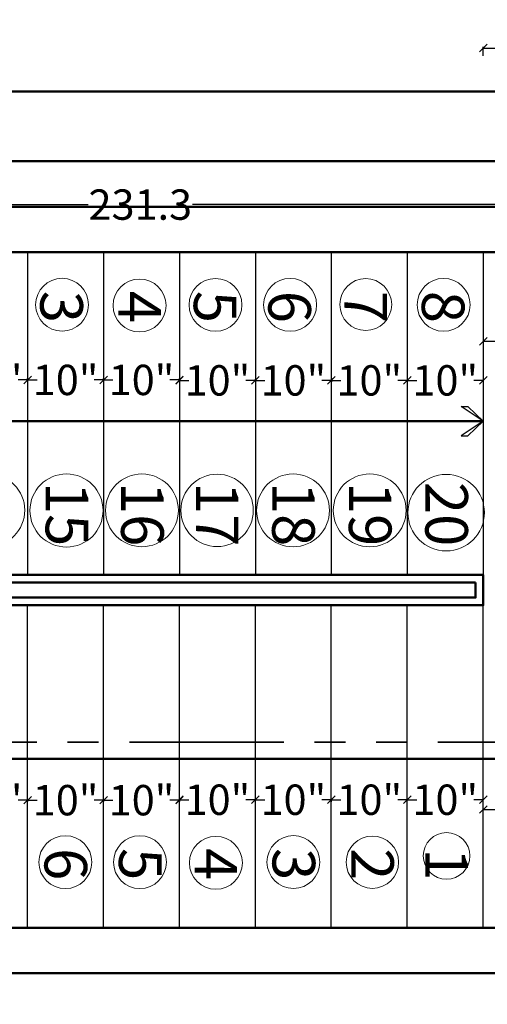
# Model space of a CAD drawing. Units: inches. Extents: x -60 to 284, y -245 to 257.
# Tile 8 of 10: x 99 to 160, y 12 to 141. Entities that reach past the tile are written whole.
import ezdxf

# ---------------------------------------------------------------- set-up
doc = ezdxf.new("R2010")
doc.units = ezdxf.units.IN
doc.header["$LTSCALE"] = 0.8
doc.header["$MEASUREMENT"] = 0
doc.linetypes.add('PHANTOM', pattern=[63.5, 31.75, -6.35, 6.35, -6.35, 6.35, -6.35])
for name, color, linetype, lineweight in [('A-ANNO-DIMS', 2, 'Continuous', 18), ('A-ANNO-SECT', 1, 'PHANTOM', 35), ('A-ANNO-SYMB', 3, 'Continuous', 18), ('A-ANNO-TEXT', 3, 'Continuous', 18), ('A-ANNO-TTLB', 7, 'Continuous', 50), ('A-FLOR-STRS', 4, 'Continuous', 25), ('A-WALL', 7, 'Continuous', 50)]:
    doc.layers.add(name, color=color, linetype=linetype, lineweight=lineweight)
doc.styles.get("Standard").update_dxf_attribs({"font": 'arial.ttf'})
doc.dimstyles.get("Standard").update_dxf_attribs({"dimtxt": 4, "dimasz": 1, "dimexe": 0.18, "dimexo": 0.0625, "dimgap": 0.09, "dimtad": 0, "dimtih": 1, "dimtoh": 1, "dimzin": 0, "dimdsep": 46, "dimlunit": 4, "dimtxsty": 'Standard', "dimblk": 'OBLIQUE', "dimcen": 0.09, "dimadec": 0, "dimazin": 0, "dimtfac": 1, "dimtofl": 0, "dimtmove": 0, "dimatfit": 3, "dimfxl": 1, "dimfxlon": 1, "dimtolj": 1, "dimtzin": 0, "dimarcsym": 0})

# ---------------------------------------------------------------- blocks, each defined once
blk = doc.blocks.new('_Oblique')
at = {"color": 0, "linetype": 'ByBlock', "lineweight": -2}
blk.add_line((-0.5, -0.5), (0.5, 0.5), dxfattribs=at)
blk = doc.blocks.new('*D1')
at = {"layer": 'A-ANNO-DIMS', "color": 0, "lineweight": -2, "ltscale": 0.8, "transparency": 16777216}
for p, q in [((149.94, 37.65), (149.94, 38.72)), ((149.94, 38.54), (151.18, 38.54)), ((159.94, 38.54), (158.69, 38.54)), ((159.94, 37.65), (159.94, 38.72))]:
    blk.add_line(p, q, dxfattribs=at)
at = {"layer": 'Defpoints', "color": 0, "ltscale": 0.8, "transparency": 16777216}
for p in [(149.94, 38.54), (149.94, 37.59), (159.94, 37.59)]:
    blk.add_point(p, dxfattribs=at)
at = {"layer": 'A-ANNO-DIMS', "color": 0, "lineweight": -2, "ltscale": 0.8, "transparency": 16777216, "rotation": 180}
blk.add_blockref('_Oblique', (149.94, 38.54), dxfattribs=at)
at = {"layer": 'A-ANNO-DIMS', "color": 0, "lineweight": -2, "ltscale": 0.8, "transparency": 16777216}
blk.add_blockref('_Oblique', (159.94, 38.54), dxfattribs=at)
at = {"layer": 'A-ANNO-DIMS', "color": 0, "ltscale": 0.8, "transparency": 16777216, "insert": (154.94, 38.54), "char_height": 4, "attachment_point": 5}
blk.add_mtext('\\A1;10"', dxfattribs=at)
blk = doc.blocks.new('*D3')
at = {"layer": 'A-ANNO-DIMS', "color": 0, "lineweight": -2, "ltscale": 0.8, "transparency": 16777216}
for p, q in [((139.94, 38.25), (139.94, 38.72)), ((139.94, 38.54), (141.18, 38.54)), ((149.94, 38.54), (148.69, 38.54)), ((149.94, 38.25), (149.94, 38.72))]:
    blk.add_line(p, q, dxfattribs=at)
at = {"layer": 'Defpoints', "color": 0, "ltscale": 0.8, "transparency": 16777216}
for p in [(139.94, 38.54), (139.94, 38.18), (149.94, 38.18)]:
    blk.add_point(p, dxfattribs=at)
at = {"layer": 'A-ANNO-DIMS', "color": 0, "lineweight": -2, "ltscale": 0.8, "transparency": 16777216, "rotation": 180}
blk.add_blockref('_Oblique', (139.94, 38.54), dxfattribs=at)
at = {"layer": 'A-ANNO-DIMS', "color": 0, "lineweight": -2, "ltscale": 0.8, "transparency": 16777216}
blk.add_blockref('_Oblique', (149.94, 38.54), dxfattribs=at)
at = {"layer": 'A-ANNO-DIMS', "color": 0, "ltscale": 0.8, "transparency": 16777216, "insert": (144.94, 38.54), "char_height": 4, "attachment_point": 5}
blk.add_mtext('\\A1;10"', dxfattribs=at)
blk = doc.blocks.new('*D4')
at = {"layer": 'A-ANNO-DIMS', "color": 0, "lineweight": -2, "ltscale": 0.8, "transparency": 16777216}
for p, q in [((129.94, 38.54), (129.94, 38.72)), ((129.94, 38.54), (131.18, 38.54)), ((139.94, 38.54), (138.69, 38.54)), ((139.94, 38.54), (139.94, 38.72))]:
    blk.add_line(p, q, dxfattribs=at)
at = {"layer": 'Defpoints', "color": 0, "ltscale": 0.8, "transparency": 16777216}
for p in [(129.94, 38.54), (139.94, 38.54), (139.94, 38.48)]:
    blk.add_point(p, dxfattribs=at)
at = {"layer": 'A-ANNO-DIMS', "color": 0, "lineweight": -2, "ltscale": 0.8, "transparency": 16777216, "rotation": 180}
blk.add_blockref('_Oblique', (129.94, 38.54), dxfattribs=at)
at = {"layer": 'A-ANNO-DIMS', "color": 0, "lineweight": -2, "ltscale": 0.8, "transparency": 16777216}
blk.add_blockref('_Oblique', (139.94, 38.54), dxfattribs=at)
at = {"layer": 'A-ANNO-DIMS', "color": 0, "ltscale": 0.8, "transparency": 16777216, "insert": (134.94, 38.54), "char_height": 4, "attachment_point": 5}
blk.add_mtext('\\A1;10"', dxfattribs=at)
blk = doc.blocks.new('*D5')
at = {"layer": 'A-ANNO-DIMS', "color": 0, "lineweight": -2, "ltscale": 0.8, "transparency": 16777216}
for p, q in [((119.94, 38.24), (119.94, 38.72)), ((119.94, 38.54), (121.18, 38.54)), ((129.94, 38.54), (128.69, 38.54)), ((129.94, 38.24), (129.94, 38.72))]:
    blk.add_line(p, q, dxfattribs=at)
at = {"layer": 'Defpoints', "color": 0, "ltscale": 0.8, "transparency": 16777216}
for p in [(119.94, 38.18), (129.94, 38.54), (129.94, 38.18)]:
    blk.add_point(p, dxfattribs=at)
at = {"layer": 'A-ANNO-DIMS', "color": 0, "lineweight": -2, "ltscale": 0.8, "transparency": 16777216, "rotation": 180}
blk.add_blockref('_Oblique', (119.94, 38.54), dxfattribs=at)
at = {"layer": 'A-ANNO-DIMS', "color": 0, "lineweight": -2, "ltscale": 0.8, "transparency": 16777216}
blk.add_blockref('_Oblique', (129.94, 38.54), dxfattribs=at)
at = {"layer": 'A-ANNO-DIMS', "color": 0, "ltscale": 0.8, "transparency": 16777216, "insert": (124.94, 38.54), "char_height": 4, "attachment_point": 5}
blk.add_mtext('\\A1;10"', dxfattribs=at)
blk = doc.blocks.new('*D6')
at = {"layer": 'A-ANNO-DIMS', "color": 0, "lineweight": -2, "ltscale": 0.8, "transparency": 16777216}
for p, q in [((109.94, 38.48), (109.94, 38.3)), ((109.94, 38.48), (111.18, 38.48)), ((119.94, 38.48), (118.69, 38.48)), ((119.94, 38.48), (119.94, 38.3))]:
    blk.add_line(p, q, dxfattribs=at)
at = {"layer": 'Defpoints', "color": 0, "ltscale": 0.8, "transparency": 16777216}
for p in [(109.94, 38.54), (119.94, 38.54), (119.94, 38.48)]:
    blk.add_point(p, dxfattribs=at)
at = {"layer": 'A-ANNO-DIMS', "color": 0, "lineweight": -2, "ltscale": 0.8, "transparency": 16777216, "rotation": 180}
blk.add_blockref('_Oblique', (109.94, 38.48), dxfattribs=at)
at = {"layer": 'A-ANNO-DIMS', "color": 0, "lineweight": -2, "ltscale": 0.8, "transparency": 16777216}
blk.add_blockref('_Oblique', (119.94, 38.48), dxfattribs=at)
at = {"layer": 'A-ANNO-DIMS', "color": 0, "ltscale": 0.8, "transparency": 16777216, "insert": (114.94, 38.48), "char_height": 4, "attachment_point": 5}
blk.add_mtext('\\A1;10"', dxfattribs=at)
blk = doc.blocks.new('*D7')
at = {"layer": 'A-ANNO-DIMS', "color": 0, "lineweight": -2, "ltscale": 0.8, "transparency": 16777216}
for p, q in [((99.94, 38.48), (99.94, 38.66)), ((99.94, 38.48), (101.18, 38.48)), ((109.94, 38.48), (108.69, 38.48)), ((109.94, 38.45), (109.94, 38.66))]:
    blk.add_line(p, q, dxfattribs=at)
at = {"layer": 'Defpoints', "color": 0, "ltscale": 0.8, "transparency": 16777216}
for p in [(99.94, 38.48), (109.94, 38.48), (109.94, 38.39)]:
    blk.add_point(p, dxfattribs=at)
at = {"layer": 'A-ANNO-DIMS', "color": 0, "lineweight": -2, "ltscale": 0.8, "transparency": 16777216, "rotation": 180}
blk.add_blockref('_Oblique', (99.94, 38.48), dxfattribs=at)
at = {"layer": 'A-ANNO-DIMS', "color": 0, "lineweight": -2, "ltscale": 0.8, "transparency": 16777216}
blk.add_blockref('_Oblique', (109.94, 38.48), dxfattribs=at)
at = {"layer": 'A-ANNO-DIMS', "color": 0, "ltscale": 0.8, "transparency": 16777216, "insert": (104.94, 38.48), "char_height": 4, "attachment_point": 5}
blk.add_mtext('\\A1;10"', dxfattribs=at)
blk = doc.blocks.new('*D8')
at = {"layer": 'A-ANNO-DIMS', "color": 0, "lineweight": -2, "ltscale": 0.8, "transparency": 16777216}
for p, q in [((89.94, 38.48), (89.94, 38.66)), ((89.94, 38.48), (91.18, 38.48)), ((99.94, 38.48), (98.69, 38.48)), ((99.94, 38.6), (99.94, 38.3))]:
    blk.add_line(p, q, dxfattribs=at)
at = {"layer": 'Defpoints', "color": 0, "ltscale": 0.8, "transparency": 16777216}
for p in [(89.94, 38.48), (99.94, 38.66), (99.94, 38.48)]:
    blk.add_point(p, dxfattribs=at)
at = {"layer": 'A-ANNO-DIMS', "color": 0, "lineweight": -2, "ltscale": 0.8, "transparency": 16777216, "rotation": 180}
blk.add_blockref('_Oblique', (89.94, 38.48), dxfattribs=at)
at = {"layer": 'A-ANNO-DIMS', "color": 0, "lineweight": -2, "ltscale": 0.8, "transparency": 16777216}
blk.add_blockref('_Oblique', (99.94, 38.48), dxfattribs=at)
at = {"layer": 'A-ANNO-DIMS', "color": 0, "ltscale": 0.8, "transparency": 16777216, "insert": (94.94, 38.48), "char_height": 4, "attachment_point": 5}
blk.add_mtext('\\A1;10"', dxfattribs=at)
blk = doc.blocks.new('*D12')
at = {"layer": 'A-ANNO-DIMS', "color": 0, "lineweight": -2, "ltscale": 0.8, "transparency": 16777216}
for p, q in [((149.94, 94.68), (149.94, 93.61)), ((149.94, 93.79), (151.18, 93.79)), ((159.94, 93.79), (158.69, 93.79)), ((159.94, 94.68), (159.94, 93.61))]:
    blk.add_line(p, q, dxfattribs=at)
at = {"layer": 'Defpoints', "color": 0, "ltscale": 0.8, "transparency": 16777216}
for p in [(149.94, 94.74), (159.94, 94.74), (149.94, 93.79)]:
    blk.add_point(p, dxfattribs=at)
at = {"layer": 'A-ANNO-DIMS', "color": 0, "lineweight": -2, "ltscale": 0.8, "transparency": 16777216, "rotation": 180}
blk.add_blockref('_Oblique', (149.94, 93.79), dxfattribs=at)
at = {"layer": 'A-ANNO-DIMS', "color": 0, "lineweight": -2, "ltscale": 0.8, "transparency": 16777216}
blk.add_blockref('_Oblique', (159.94, 93.79), dxfattribs=at)
at = {"layer": 'A-ANNO-DIMS', "color": 0, "ltscale": 0.8, "transparency": 16777216, "insert": (154.94, 93.79), "char_height": 4, "attachment_point": 5}
blk.add_mtext('\\A1;10"', dxfattribs=at)
blk = doc.blocks.new('*D13')
at = {"layer": 'A-ANNO-DIMS', "color": 0, "lineweight": -2, "ltscale": 0.8, "transparency": 16777216}
for p, q in [((139.94, 94.09), (139.94, 93.61)), ((139.94, 93.79), (141.18, 93.79)), ((149.94, 93.79), (148.69, 93.79)), ((149.94, 94.09), (149.94, 93.61))]:
    blk.add_line(p, q, dxfattribs=at)
at = {"layer": 'Defpoints', "color": 0, "ltscale": 0.8, "transparency": 16777216}
for p in [(139.94, 94.15), (139.94, 93.79), (149.94, 94.15)]:
    blk.add_point(p, dxfattribs=at)
at = {"layer": 'A-ANNO-DIMS', "color": 0, "lineweight": -2, "ltscale": 0.8, "transparency": 16777216, "rotation": 180}
blk.add_blockref('_Oblique', (139.94, 93.79), dxfattribs=at)
at = {"layer": 'A-ANNO-DIMS', "color": 0, "lineweight": -2, "ltscale": 0.8, "transparency": 16777216}
blk.add_blockref('_Oblique', (149.94, 93.79), dxfattribs=at)
at = {"layer": 'A-ANNO-DIMS', "color": 0, "ltscale": 0.8, "transparency": 16777216, "insert": (144.94, 93.79), "char_height": 4, "attachment_point": 5}
blk.add_mtext('\\A1;10"', dxfattribs=at)
blk = doc.blocks.new('*D14')
at = {"layer": 'A-ANNO-DIMS', "color": 0, "lineweight": -2, "ltscale": 0.8, "transparency": 16777216}
for p, q in [((129.94, 93.79), (129.94, 93.97)), ((129.94, 93.79), (131.18, 93.79)), ((139.94, 93.79), (138.69, 93.79)), ((139.94, 93.79), (139.94, 93.61))]:
    blk.add_line(p, q, dxfattribs=at)
at = {"layer": 'Defpoints', "color": 0, "ltscale": 0.8, "transparency": 16777216}
for p in [(129.94, 93.79), (139.94, 93.85), (139.94, 93.79)]:
    blk.add_point(p, dxfattribs=at)
at = {"layer": 'A-ANNO-DIMS', "color": 0, "lineweight": -2, "ltscale": 0.8, "transparency": 16777216, "rotation": 180}
blk.add_blockref('_Oblique', (129.94, 93.79), dxfattribs=at)
at = {"layer": 'A-ANNO-DIMS', "color": 0, "lineweight": -2, "ltscale": 0.8, "transparency": 16777216}
blk.add_blockref('_Oblique', (139.94, 93.79), dxfattribs=at)
at = {"layer": 'A-ANNO-DIMS', "color": 0, "ltscale": 0.8, "transparency": 16777216, "insert": (134.94, 93.79), "char_height": 4, "attachment_point": 5}
blk.add_mtext('\\A1;10"', dxfattribs=at)
blk = doc.blocks.new('*D15')
at = {"layer": 'A-ANNO-DIMS', "color": 0, "lineweight": -2, "ltscale": 0.8, "transparency": 16777216}
for p, q in [((119.94, 94.09), (119.94, 93.61)), ((119.94, 93.79), (121.18, 93.79)), ((129.94, 93.79), (128.69, 93.79)), ((129.94, 94.09), (129.94, 93.61))]:
    blk.add_line(p, q, dxfattribs=at)
at = {"layer": 'Defpoints', "color": 0, "ltscale": 0.8, "transparency": 16777216}
for p in [(119.94, 94.15), (129.94, 94.15), (129.94, 93.79)]:
    blk.add_point(p, dxfattribs=at)
at = {"layer": 'A-ANNO-DIMS', "color": 0, "lineweight": -2, "ltscale": 0.8, "transparency": 16777216, "rotation": 180}
blk.add_blockref('_Oblique', (119.94, 93.79), dxfattribs=at)
at = {"layer": 'A-ANNO-DIMS', "color": 0, "lineweight": -2, "ltscale": 0.8, "transparency": 16777216}
blk.add_blockref('_Oblique', (129.94, 93.79), dxfattribs=at)
at = {"layer": 'A-ANNO-DIMS', "color": 0, "ltscale": 0.8, "transparency": 16777216, "insert": (124.94, 93.79), "char_height": 4, "attachment_point": 5}
blk.add_mtext('\\A1;10"', dxfattribs=at)
blk = doc.blocks.new('*D16')
at = {"layer": 'A-ANNO-DIMS', "color": 0, "lineweight": -2, "ltscale": 0.8, "transparency": 16777216}
for p, q in [((109.94, 93.85), (109.94, 94.03)), ((109.94, 93.85), (111.18, 93.85)), ((119.94, 93.85), (118.69, 93.85)), ((119.94, 93.85), (119.94, 94.03))]:
    blk.add_line(p, q, dxfattribs=at)
at = {"layer": 'Defpoints', "color": 0, "ltscale": 0.8, "transparency": 16777216}
for p in [(109.94, 93.79), (119.94, 93.85), (119.94, 93.79)]:
    blk.add_point(p, dxfattribs=at)
at = {"layer": 'A-ANNO-DIMS', "color": 0, "lineweight": -2, "ltscale": 0.8, "transparency": 16777216, "rotation": 180}
blk.add_blockref('_Oblique', (109.94, 93.85), dxfattribs=at)
at = {"layer": 'A-ANNO-DIMS', "color": 0, "lineweight": -2, "ltscale": 0.8, "transparency": 16777216}
blk.add_blockref('_Oblique', (119.94, 93.85), dxfattribs=at)
at = {"layer": 'A-ANNO-DIMS', "color": 0, "ltscale": 0.8, "transparency": 16777216, "insert": (114.94, 93.85), "char_height": 4, "attachment_point": 5}
blk.add_mtext('\\A1;10"', dxfattribs=at)
blk = doc.blocks.new('*D17')
at = {"layer": 'A-ANNO-DIMS', "color": 0, "lineweight": -2, "ltscale": 0.8, "transparency": 16777216}
for p, q in [((99.94, 93.85), (99.94, 94.03)), ((99.94, 93.85), (101.18, 93.85)), ((109.94, 93.85), (108.69, 93.85)), ((109.94, 93.88), (109.94, 93.67))]:
    blk.add_line(p, q, dxfattribs=at)
at = {"layer": 'Defpoints', "color": 0, "ltscale": 0.8, "transparency": 16777216}
for p in [(99.94, 93.85), (109.94, 93.94), (109.94, 93.85)]:
    blk.add_point(p, dxfattribs=at)
at = {"layer": 'A-ANNO-DIMS', "color": 0, "lineweight": -2, "ltscale": 0.8, "transparency": 16777216, "rotation": 180}
blk.add_blockref('_Oblique', (99.94, 93.85), dxfattribs=at)
at = {"layer": 'A-ANNO-DIMS', "color": 0, "lineweight": -2, "ltscale": 0.8, "transparency": 16777216}
blk.add_blockref('_Oblique', (109.94, 93.85), dxfattribs=at)
at = {"layer": 'A-ANNO-DIMS', "color": 0, "ltscale": 0.8, "transparency": 16777216, "insert": (104.94, 93.85), "char_height": 4, "attachment_point": 5}
blk.add_mtext('\\A1;10"', dxfattribs=at)
blk = doc.blocks.new('*D18')
at = {"layer": 'A-ANNO-DIMS', "color": 0, "lineweight": -2, "ltscale": 0.8, "transparency": 16777216}
for p, q in [((89.94, 93.85), (89.94, 94.03)), ((89.94, 93.85), (91.18, 93.85)), ((99.94, 93.85), (98.69, 93.85)), ((99.94, 93.73), (99.94, 94.03))]:
    blk.add_line(p, q, dxfattribs=at)
at = {"layer": 'Defpoints', "color": 0, "ltscale": 0.8, "transparency": 16777216}
for p in [(89.94, 93.85), (99.94, 93.85), (99.94, 93.67)]:
    blk.add_point(p, dxfattribs=at)
at = {"layer": 'A-ANNO-DIMS', "color": 0, "lineweight": -2, "ltscale": 0.8, "transparency": 16777216, "rotation": 180}
blk.add_blockref('_Oblique', (89.94, 93.85), dxfattribs=at)
at = {"layer": 'A-ANNO-DIMS', "color": 0, "lineweight": -2, "ltscale": 0.8, "transparency": 16777216}
blk.add_blockref('_Oblique', (99.94, 93.85), dxfattribs=at)
at = {"layer": 'A-ANNO-DIMS', "color": 0, "ltscale": 0.8, "transparency": 16777216, "insert": (94.94, 93.85), "char_height": 4, "attachment_point": 5}
blk.add_mtext('\\A1;10"', dxfattribs=at)
blk = doc.blocks.new('*D22')
at = {"layer": 'A-ANNO-DIMS', "color": 0, "lineweight": -2, "ltscale": 0.8, "transparency": 16777216}
for p, q in [((159.94, 36.25), (159.94, 37.43)), ((159.94, 37.25), (174.03, 37.25)), ((198.94, 37.25), (184.84, 37.25)), ((198.94, 36.25), (198.94, 37.43))]:
    blk.add_line(p, q, dxfattribs=at)
at = {"layer": 'Defpoints', "color": 0, "ltscale": 0.8, "transparency": 16777216}
for p in [(198.94, 37.25), (159.94, 21.67), (198.94, 21.67)]:
    blk.add_point(p, dxfattribs=at)
at = {"layer": 'A-ANNO-DIMS', "color": 0, "lineweight": -2, "ltscale": 0.8, "transparency": 16777216, "rotation": 180}
blk.add_blockref('_Oblique', (159.94, 37.25), dxfattribs=at)
at = {"layer": 'A-ANNO-DIMS', "color": 0, "lineweight": -2, "ltscale": 0.8, "transparency": 16777216}
blk.add_blockref('_Oblique', (198.94, 37.25), dxfattribs=at)
at = {"layer": 'A-ANNO-DIMS', "color": 0, "ltscale": 0.8, "transparency": 16777216, "insert": (179.44, 37.25), "char_height": 4, "attachment_point": 5}
blk.add_mtext('\\A1;3\'-3"', dxfattribs=at)
blk = doc.blocks.new('*D23')
at = {"layer": 'A-ANNO-DIMS', "color": 0, "lineweight": -2, "ltscale": 0.8, "transparency": 16777216}
for p, q in [((159.94, 99.95), (159.94, 98.77)), ((198.94, 99.95), (198.94, 98.77)), ((159.94, 98.95), (174.03, 98.95)), ((198.94, 98.95), (184.84, 98.95))]:
    blk.add_line(p, q, dxfattribs=at)
at = {"layer": 'Defpoints', "color": 0, "ltscale": 0.8, "transparency": 16777216}
for p in [(159.94, 110.67), (198.94, 110.67), (198.94, 98.95)]:
    blk.add_point(p, dxfattribs=at)
at = {"layer": 'A-ANNO-DIMS', "color": 0, "lineweight": -2, "ltscale": 0.8, "transparency": 16777216, "rotation": 180}
blk.add_blockref('_Oblique', (159.94, 98.95), dxfattribs=at)
at = {"layer": 'A-ANNO-DIMS', "color": 0, "lineweight": -2, "ltscale": 0.8, "transparency": 16777216}
blk.add_blockref('_Oblique', (198.94, 98.95), dxfattribs=at)
at = {"layer": 'A-ANNO-DIMS', "color": 0, "ltscale": 0.8, "transparency": 16777216, "insert": (179.44, 98.95), "char_height": 4, "attachment_point": 5}
blk.add_mtext('\\A1;3\'-3"', dxfattribs=at)
blk = doc.blocks.new('*D76')
at = {"layer": 'A-ANNO-DIMS', "color": 0, "lineweight": -2, "ltscale": 0.8, "transparency": 16777216}
for p, q in [((-0.88, 117.95), (-0.88, 116.77)), ((-0.88, 116.95), (107.9, 116.95)), ((230.43, 116.95), (121.65, 116.95)), ((230.43, 117.95), (230.43, 116.77))]:
    blk.add_line(p, q, dxfattribs=at)
at = {"layer": 'Defpoints', "color": 0, "ltscale": 0.8, "transparency": 16777216}
for p in [(-0.88, 131.85), (230.43, 131.85), (230.43, 116.95)]:
    blk.add_point(p, dxfattribs=at)
at = {"layer": 'A-ANNO-DIMS', "color": 0, "lineweight": -2, "ltscale": 0.8, "transparency": 16777216, "rotation": 180}
blk.add_blockref('_Oblique', (-0.88, 116.95), dxfattribs=at)
at = {"layer": 'A-ANNO-DIMS', "color": 0, "lineweight": -2, "ltscale": 0.8, "transparency": 16777216}
blk.add_blockref('_Oblique', (230.43, 116.95), dxfattribs=at)
at = {"layer": 'A-ANNO-DIMS', "color": 0, "ltscale": 0.8, "transparency": 16777216, "insert": (114.78, 116.95), "char_height": 4, "attachment_point": 5}
blk.add_mtext('\\A1;231.3', dxfattribs=at)
blk = doc.blocks.new('*D95')
at = {"layer": 'A-ANNO-DIMS', "color": 0, "lineweight": -2, "ltscale": 0.8, "transparency": 16777216}
for p, q in [((159.94, 136.57), (159.94, 137.75)), ((159.94, 137.57), (165.41, 137.57)), ((187.74, 137.57), (182.26, 137.57)), ((187.74, 136.57), (187.74, 137.75))]:
    blk.add_line(p, q, dxfattribs=at)
at = {"layer": 'Defpoints', "color": 0, "ltscale": 0.8, "transparency": 16777216}
for p in [(187.74, 137.57), (159.94, 110.67), (187.74, 107.67)]:
    blk.add_point(p, dxfattribs=at)
at = {"layer": 'A-ANNO-DIMS', "color": 0, "lineweight": -2, "ltscale": 0.8, "transparency": 16777216, "rotation": 180}
blk.add_blockref('_Oblique', (159.94, 137.57), dxfattribs=at)
at = {"layer": 'A-ANNO-DIMS', "color": 0, "lineweight": -2, "ltscale": 0.8, "transparency": 16777216}
blk.add_blockref('_Oblique', (187.74, 137.57), dxfattribs=at)
at = {"layer": 'A-ANNO-DIMS', "color": 0, "ltscale": 0.8, "transparency": 16777216, "insert": (173.84, 137.57), "char_height": 4, "attachment_point": 5}
blk.add_mtext('\\A1;27.806', dxfattribs=at)

msp = doc.modelspace()

# ---------------------------------------------------------------- linework, layer by layer
at = {"layer": 'A-ANNO-SECT', "ltscale": 0.8}
msp.add_line((255.5807, 46.116), (-23.5489, 46.116), dxfattribs=at)
at = {"layer": 'A-ANNO-SYMB', "ltscale": 0.8}
for centre, radius in [((104.4744, 103.7611), 3.4782), ((114.6823, 103.6578), 3.4851), ((124.683, 103.7381), 3.4796), ((134.5041, 103.7458), 3.485), ((144.4694, 103.7821), 3.4155), ((154.7246, 103.7496), 3.4829), ((94.8158, 76.6775), 4.7576), ((105.0612, 76.645), 4.8123), ((115.0001, 76.6679), 4.7941), ((124.8945, 76.666), 4.7667), ((134.8957, 76.6603), 4.8002), ((144.9934, 76.6603), 4.8002), ((155.0585, 76.364), 5.0387), ((104.9093, 30.3161), 3.485), ((114.7305, 30.3085), 3.4796), ((134.9391, 30.3314), 3.4782), ((145.3428, 30.3104), 3.4482), ((155.1063, 31.1342), 3.069), ((124.7312, 30.2282), 3.4851)]:
    msp.add_circle(centre, radius, dxfattribs=at)
at = {"layer": 'A-ANNO-TTLB', "ltscale": 0.8}
for points in [[(-0.8787, 239.5184), (230.4297, 239.5184), (230.4297, 131.8542), (-0.8787, 131.8542)], [(0.0867, 122.666), (239.6639, 122.666), (239.6639, 9.666), (0.0867, 9.666)]]:
    msp.add_lwpolyline(points, close=True, dxfattribs=at)
at = {"layer": 'A-FLOR-STRS'}
for p, q in [((99.9361, 110.666), (99.9361, 68.166)), ((109.9361, 110.666), (109.9361, 68.166)), ((119.9361, 110.666), (119.9361, 68.166)), ((129.9361, 110.666), (129.9361, 68.166)), ((139.9361, 110.666), (139.9361, 68.166)), ((149.9361, 110.666), (149.9361, 68.166)), ((159.9361, 110.666), (159.9361, 66.166)), ((159.9361, 21.666), (159.9361, 66.166)), ((99.9361, 21.666), (99.9361, 64.166)), ((109.9361, 21.666), (109.9361, 64.166)), ((119.9361, 21.666), (119.9361, 64.166)), ((129.9361, 21.666), (129.9361, 64.166)), ((139.9361, 21.666), (139.9361, 64.166)), ((149.9361, 21.666), (149.9361, 64.166))]:
    msp.add_line(p, q, dxfattribs=at)
at = {"layer": 'A-FLOR-STRS', "ltscale": 0.8}
for p, q in [((157.0555, 90.33), (157.8917, 90.3572)), ((159.9361, 88.416), (157.0555, 90.33)), ((157.8917, 90.3572), (159.9361, 88.416)), ((159.9361, 88.416), (157.0555, 86.5021)), ((157.8917, 86.4749), (159.9361, 88.416)), ((157.0555, 86.5021), (157.8917, 86.4749))]:
    msp.add_line(p, q, dxfattribs=at)
at = {"layer": 'A-WALL', "ltscale": 0.8}
for p, q in [((69.9361, 88.416), (159.9361, 88.416)), ((168.271, 43.916), (43.6123, 43.916))]:
    msp.add_line(p, q, dxfattribs=at)
at = {"layer": 'A-WALL'}
for points in [[(198.9361, 116.666), (198.9361, 110.666), (159.9361, 110.666), (79.9361, 110.666), (37.9361, 110.666), (27.9361, 110.666), (27.9361, 122.666)], [(192.9361, 116.666), (159.9361, 116.666), (79.9361, 116.666), (37.9361, 116.666), (33.9361, 116.666), (33.9361, 122.666)], [(198.9361, 9.666), (198.9361, 21.666), (159.9361, 21.666), (79.9361, 21.666), (37.9361, 21.666), (27.9361, 21.666), (27.9361, 9.666)], [(192.9361, 9.666), (192.9361, 15.666), (159.9361, 15.666), (79.9361, 15.666), (37.9361, 15.666), (33.9361, 15.666), (33.9361, 9.666)]]:
    msp.add_lwpolyline(points, dxfattribs=at)
for points in [[(159.9361, 68.166), (69.9361, 68.166), (69.9361, 64.166), (159.9361, 64.166)], [(158.9361, 67.166), (70.9361, 67.166), (70.9361, 65.166), (158.9361, 65.166)]]:
    msp.add_lwpolyline(points, close=True, dxfattribs=at)

# ---------------------------------------------------------------- texts
at = {"layer": 'A-ANNO-TEXT', "ltscale": 0.8, "rotation": 270}
for s, insert, char_height, attachment_point in [('3', (101.6111, 105.596), 5.6042, 7), ('4', (111.8802, 105.596), 5.6042, 7), ('5', (121.8331, 105.596), 5.6042, 7), ('6', (131.6428, 105.596), 5.6042, 7), ('7', (141.6673, 105.596), 5.6042, 7), ('8', (151.8633, 105.596), 5.6042, 7), ('15', (107.9225, 80.4161), 5.60417, 1), ('16', (117.8614, 80.4161), 5.60417, 1), ('17', (127.7081, 80.4161), 5.60417, 1), ('18', (137.757, 80.4161), 5.60417, 1), ('19', (147.8547, 80.4161), 5.60417, 1), ('20', (157.9199, 80.4161), 5.60417, 1), ('6', (107.7707, 32.1663), 5.6042, 1), ('5', (117.5804, 32.1663), 5.6042, 1), ('4', (127.5333, 32.1663), 5.6042, 1), ('3', (137.8023, 32.1663), 5.6042, 1), ('2', (148.1564, 32.1663), 5.6042, 1), ('1', (157.9199, 32.1663), 5.6042, 1)]:
    msp.add_mtext_dynamic_manual_height_columns(s, width=28.020867, gutter_width=2.8021, heights=[0], dxfattribs=dict(at, insert=insert, char_height=char_height, attachment_point=attachment_point))

# ---------------------------------------------------------------- dimensions: what is measured, and where the dimension line sits
at = {"layer": 'A-ANNO-DIMS', "ltscale": 0.8}
for base, p1, p2, override, picture, middle in [((187.74258, 137.56605), (159.93611, 110.66605), (187.74258, 107.66605), {"dimdec": 3, "dimlfac": 1, "dimrnd": 0, "dimzin": 0, "dimdsep": 46, "dimlunit": 2}, '*D95', (173.83935, 137.56605)), ((230.4297, 116.9542), (-0.8787, 131.8542), (230.4297, 131.8542), {"dimdec": 1, "dimlfac": 1, "dimrnd": 0, "dimzin": 0, "dimdsep": 46, "dimlunit": 2}, '*D76', (114.7755, 116.9542)), ((198.9361, 98.9541), (159.9361, 110.666), (198.9361, 110.666), {"dimclrd": 0, "dimclre": 0, "dimclrt": 0}, '*D23', (179.4361, 98.9541)), ((99.9361, 93.8517), (89.9361, 93.8517), (99.9361, 93.6717), {"dimclrd": 0, "dimclre": 0, "dimclrt": 0}, '*D18', (94.9361, 93.8517)), ((109.9361, 93.8517), (99.9361, 93.8517), (109.9361, 93.9443), {"dimclrd": 0, "dimclre": 0, "dimclrt": 0}, '*D17', (104.9361, 93.8517)), ((119.9361, 93.8517), (109.9361, 93.7945), (119.9361, 93.7945), {"dimclrd": 0, "dimclre": 0, "dimclrt": 0}, '*D16', (114.9361, 93.8517)), ((129.9361, 93.7945), (119.9361, 94.1514), (129.9361, 94.1514), {"dimclrd": 0, "dimclre": 0, "dimclrt": 0}, '*D15', (124.9361, 93.7945)), ((139.9361, 93.7945), (129.9361, 93.7945), (139.9361, 93.8502), {"dimclrd": 0, "dimclre": 0, "dimclrt": 0}, '*D14', (134.9361, 93.7945)), ((139.9361, 93.7945), (149.9361, 94.1483), (139.9361, 94.1483), {"dimclrd": 0, "dimclre": 0, "dimclrt": 0}, '*D13', (144.9361, 93.7945)), ((149.9361, 93.7945), (159.9361, 94.7447), (149.9361, 94.7447), {"dimclrd": 0, "dimclre": 0, "dimclrt": 0}, '*D12', (154.9361, 93.7945)), ((99.9361, 38.4804), (89.9361, 38.4804), (99.9361, 38.6604), {"dimclrd": 0, "dimclre": 0, "dimclrt": 0}, '*D8', (94.9361, 38.4804)), ((109.9361, 38.4804), (99.9361, 38.4804), (109.9361, 38.3878), {"dimclrd": 0, "dimclre": 0, "dimclrt": 0}, '*D7', (104.9361, 38.4804)), ((119.9361, 38.4804), (109.9361, 38.5376), (119.9361, 38.5376), {"dimclrd": 0, "dimclre": 0, "dimclrt": 0}, '*D6', (114.9361, 38.4804)), ((129.9361, 38.5376), (119.9361, 38.1807), (129.9361, 38.1807), {"dimclrd": 0, "dimclre": 0, "dimclrt": 0}, '*D5', (124.9361, 38.5376)), ((139.9361, 38.5376), (129.9361, 38.5376), (139.9361, 38.4819), {"dimclrd": 0, "dimclre": 0, "dimclrt": 0}, '*D4', (134.9361, 38.5376)), ((139.9361, 38.5376), (149.9361, 38.1838), (139.9361, 38.1838), {"dimclrd": 0, "dimclre": 0, "dimclrt": 0}, '*D3', (144.9361, 38.5376)), ((149.9361, 38.5376), (159.9361, 37.5874), (149.9361, 37.5874), {"dimclrd": 0, "dimclre": 0, "dimclrt": 0}, '*D1', (154.9361, 38.5376)), ((198.9361, 37.2467), (159.9361, 21.666), (198.9361, 21.666), {"dimclrd": 0, "dimclre": 0, "dimclrt": 0}, '*D22', (179.4361, 37.2467))]:
    dim = msp.add_linear_dim(base=base, p1=p1, p2=p2, dimstyle='Standard', override=override, dxfattribs=at)
    dim.commit()
    dim.dimension.update_dxf_attribs({"geometry": picture, "text_midpoint": middle})

doc.saveas('drawing.dxf')
